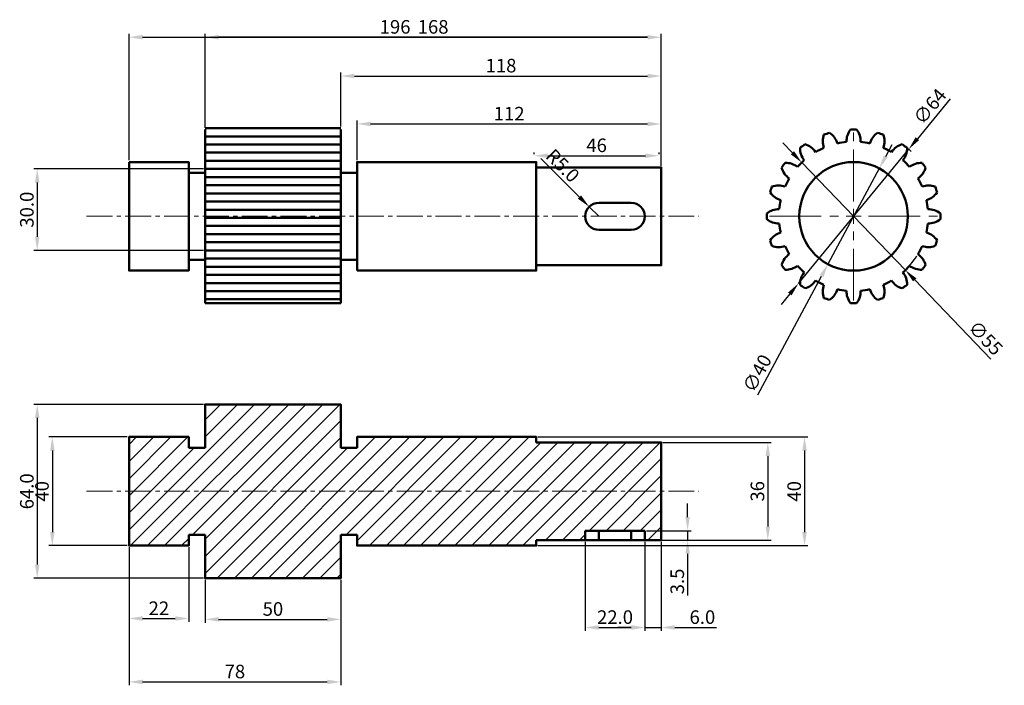
# Model space of a CAD drawing. Units: millimetres. Extents: x 2854 to 3217, y 1568 to 1813.
import ezdxf

# ---------------------------------------------------------------- set-up
doc = ezdxf.new("R2010")
doc.units = ezdxf.units.MM
doc.linetypes.add('CENTER2', pattern=[28.575, 19.05, -3.175, 3.175, -3.175])
for name, color, linetype, lineweight in [('M-CNTR', 1, 'CENTER2', 18), ('M-DIMS', 2, 'Continuous', 25), ('M-HATC', 8, 'Continuous', 18), ('M-OUTL', 7, 'Continuous', 50)]:
    doc.layers.add(name, color=color, linetype=linetype, lineweight=lineweight)
doc.styles.get("Standard").update_dxf_attribs({"font": 'arial.ttf'})
doc.dimstyles.new('ISO-25', dxfattribs={"dimtxt": 5, "dimasz": 5, "dimexe": 1.25, "dimexo": 0.625, "dimtad": 1, "dimdsep": 46, "dimtxsty": 'Standard', "dimcen": 2.5, "dimclrd": 3, "dimadec": 0, "dimazin": 0, "dimtfac": 1, "dimtmove": 0, "dimatfit": 3, "dimfxl": 1, "dimarcsym": 0})

# ---------------------------------------------------------------- blocks, each defined once
blk = doc.blocks.new('*D1')
at = {"layer": 'Defpoints', "color": 0, "transparency": 16777216}
for p in [(3090.59, 1806.21), (2894.59, 1760.27), (3090.59, 1758.27)]:
    blk.add_point(p, dxfattribs=at)
at = {"layer": 'M-DIMS', "color": 0, "lineweight": -2, "transparency": 16777216}
for p, q in [((2894.59, 1760.89), (2894.59, 1807.46)), ((2899.59, 1806.21), (3085.59, 1806.21)), ((3090.59, 1758.89), (3090.59, 1807.46))]:
    blk.add_line(p, q, dxfattribs=at)
at = {"layer": 'M-DIMS', "color": 0, "transparency": 16777216}
for points in [[(2899.59, 1807.05), (2899.59, 1805.38), (2894.59, 1806.21)], [(3085.59, 1807.05), (3085.59, 1805.38), (3090.59, 1806.21)]]:
    blk.add_solid(points, dxfattribs=at)
at = {"layer": 'M-DIMS', "color": 0, "transparency": 16777216, "insert": (2992.59, 1809.39), "char_height": 5, "attachment_point": 5}
blk.add_mtext('196', dxfattribs=at)
blk = doc.blocks.new('*D2')
at = {"layer": 'Defpoints', "color": 0, "transparency": 16777216}
for p in [(2922.59, 1806.21), (2922.59, 1772.27), (3090.59, 1758.27)]:
    blk.add_point(p, dxfattribs=at)
at = {"layer": 'M-DIMS', "color": 0, "lineweight": -2, "transparency": 16777216}
for p, q in [((2922.59, 1772.89), (2922.59, 1807.46)), ((3085.59, 1806.21), (2927.59, 1806.21)), ((3090.59, 1758.89), (3090.59, 1807.46))]:
    blk.add_line(p, q, dxfattribs=at)
at = {"layer": 'M-DIMS', "color": 0, "transparency": 16777216}
for points in [[(2927.59, 1807.05), (2927.59, 1805.38), (2922.59, 1806.21)], [(3085.59, 1807.05), (3085.59, 1805.38), (3090.59, 1806.21)]]:
    blk.add_solid(points, dxfattribs=at)
at = {"layer": 'M-DIMS', "color": 0, "transparency": 16777216, "insert": (3006.59, 1809.39), "char_height": 5, "attachment_point": 5}
blk.add_mtext('168', dxfattribs=at)
blk = doc.blocks.new('*D3')
at = {"layer": 'Defpoints', "color": 0, "transparency": 16777216}
for p in [(3090.59, 1791.93), (2972.59, 1772.72), (3090.59, 1772.72)]:
    blk.add_point(p, dxfattribs=at)
at = {"layer": 'M-DIMS', "color": 0, "lineweight": -2, "transparency": 16777216}
for p, q in [((2972.59, 1773.34), (2972.59, 1793.18)), ((2977.59, 1791.93), (3085.59, 1791.93)), ((3090.59, 1773.34), (3090.59, 1793.18))]:
    blk.add_line(p, q, dxfattribs=at)
at = {"layer": 'M-DIMS', "color": 0, "transparency": 16777216}
for points in [[(2977.59, 1792.77), (2977.59, 1791.1), (2972.59, 1791.93)], [(3085.59, 1792.77), (3085.59, 1791.1), (3090.59, 1791.93)]]:
    blk.add_solid(points, dxfattribs=at)
at = {"layer": 'M-DIMS', "color": 0, "transparency": 16777216, "insert": (3031.59, 1795.11), "char_height": 5, "attachment_point": 5}
blk.add_mtext('118', dxfattribs=at)
blk = doc.blocks.new('*D4')
at = {"layer": 'Defpoints', "color": 0, "transparency": 16777216}
for p in [(3090.59, 1774.28), (2978.59, 1760.27), (3090.59, 1760.27)]:
    blk.add_point(p, dxfattribs=at)
at = {"layer": 'M-DIMS', "color": 0, "lineweight": -2, "transparency": 16777216}
for p, q in [((2978.59, 1760.89), (2978.59, 1775.53)), ((2983.59, 1774.28), (3085.59, 1774.28)), ((3090.59, 1760.89), (3090.59, 1775.53))]:
    blk.add_line(p, q, dxfattribs=at)
at = {"layer": 'M-DIMS', "color": 0, "transparency": 16777216}
for points in [[(2983.59, 1775.12), (2983.59, 1773.45), (2978.59, 1774.28)], [(3085.59, 1775.12), (3085.59, 1773.45), (3090.59, 1774.28)]]:
    blk.add_solid(points, dxfattribs=at)
at = {"layer": 'M-DIMS', "color": 0, "transparency": 16777216, "insert": (3034.59, 1777.42), "char_height": 5, "attachment_point": 5}
blk.add_mtext('112', dxfattribs=at)
blk = doc.blocks.new('*D5')
at = {"layer": 'Defpoints', "color": 0, "transparency": 16777216}
for p in [(3043.81, 1762.58), (3089.81, 1762.58), (3089.81, 1762.58)]:
    blk.add_point(p, dxfattribs=at)
at = {"layer": 'M-DIMS', "color": 0, "lineweight": -2, "transparency": 16777216}
for p, q in [((3043.81, 1763.21), (3043.81, 1763.83)), ((3048.81, 1762.58), (3084.81, 1762.58)), ((3089.81, 1763.21), (3089.81, 1763.83))]:
    blk.add_line(p, q, dxfattribs=at)
at = {"layer": 'M-DIMS', "color": 0, "transparency": 16777216}
for points in [[(3048.81, 1763.42), (3048.81, 1761.75), (3043.81, 1762.58)], [(3084.81, 1763.42), (3084.81, 1761.75), (3089.81, 1762.58)]]:
    blk.add_solid(points, dxfattribs=at)
at = {"layer": 'M-DIMS', "color": 0, "transparency": 16777216, "insert": (3066.81, 1765.76), "char_height": 5, "attachment_point": 5}
blk.add_mtext('46', dxfattribs=at)
blk = doc.blocks.new('*D6')
at = {"layer": 'Defpoints', "color": 0, "transparency": 16777216}
for p in [(3181.76, 1765), (3141.14, 1715.54)]:
    blk.add_point(p, dxfattribs=at)
at = {"layer": 'M-DIMS', "color": 0, "lineweight": -2, "transparency": 16777216}
for p, q in [((3197, 1783.55), (3184.93, 1768.86)), ((3141.14, 1715.54), (3181.76, 1765)), ((3137.96, 1711.68), (3134.79, 1707.81))]:
    blk.add_line(p, q, dxfattribs=at)
blk.add_arc((3161.45, 1740.27), 32, 48.3615, 50.9227, dxfattribs=at)
at = {"layer": 'M-DIMS', "color": 0, "transparency": 16777216}
for points in [[(3184.29, 1769.39), (3185.58, 1768.33), (3181.76, 1765)], [(3137.32, 1712.21), (3138.61, 1711.15), (3141.14, 1715.54)]]:
    blk.add_solid(points, dxfattribs=at)
at = {"layer": 'M-DIMS', "color": 0, "transparency": 16777216, "insert": (3190.05, 1780.31), "char_height": 5, "attachment_point": 5, "rotation": 50.5996}
blk.add_mtext('∅64', dxfattribs=at)
blk = doc.blocks.new('*U7')
at = {"layer": 'M-CNTR', "color": 0, "transparency": 16777216}
for p, q in [((0, 5.5), (0, 31)), ((-31, 0), (-5.5, 0)), ((5.5, 0), (31, 0)), ((0, -31), (0, -5.5))]:
    blk.add_line(p, q, dxfattribs=at)
at = {"layer": 'M-CNTR', "color": 0, "linetype": 'Continuous', "transparency": 16777216}
for p, q in [((-2.75, 0), (2.75, 0)), ((0, -2.75), (0, 2.75))]:
    blk.add_line(p, q, dxfattribs=at)
blk = doc.blocks.new('*U8')
at = {"layer": 'M-CNTR', "color": 0, "transparency": 16777216}
for p, q in [((0, 5.5), (0, 31)), ((-31, 0), (-5.5, 0)), ((5.5, 0), (31, 0)), ((0, -31), (0, -5.5))]:
    blk.add_line(p, q, dxfattribs=at)
at = {"layer": 'M-CNTR', "color": 0, "linetype": 'Continuous', "transparency": 16777216}
for p, q in [((-2.75, 0), (2.75, 0)), ((0, -2.75), (0, 2.75))]:
    blk.add_line(p, q, dxfattribs=at)
blk = doc.blocks.new('*D9')
at = {"layer": 'Defpoints', "color": 0, "transparency": 16777216}
for p in [(3170.9, 1757.89), (3151.99, 1722.65)]:
    blk.add_point(p, dxfattribs=at)
at = {"layer": 'M-DIMS', "color": 0, "lineweight": -2, "transparency": 16777216}
for p, q in [((3173.27, 1762.3), (3175.63, 1766.71)), ((3170.9, 1757.89), (3151.99, 1722.65)), ((3126.17, 1674.51), (3149.63, 1718.24))]:
    blk.add_line(p, q, dxfattribs=at)
at = {"layer": 'M-DIMS', "color": 0, "transparency": 16777216}
for points in [[(3172.53, 1762.69), (3174, 1761.91), (3170.9, 1757.89)], [(3148.9, 1718.63), (3150.36, 1717.85), (3151.99, 1722.65)]]:
    blk.add_solid(points, dxfattribs=at)
at = {"layer": 'M-DIMS', "color": 0, "transparency": 16777216, "insert": (3126.52, 1682.17), "char_height": 5, "attachment_point": 5, "rotation": 61.7895}
blk.add_mtext('∅40', dxfattribs=at)
blk = doc.blocks.new('*D10')
at = {"layer": 'Defpoints', "color": 0, "transparency": 16777216}
for p in [(3142.37, 1760.08), (3180.52, 1720.46)]:
    blk.add_point(p, dxfattribs=at)
at = {"layer": 'M-DIMS', "color": 0, "lineweight": -2, "transparency": 16777216}
for p, q in [((3138.91, 1763.68), (3135.44, 1767.28)), ((3142.37, 1760.08), (3180.52, 1720.46)), ((3212.03, 1687.73), (3183.99, 1716.86))]:
    blk.add_line(p, q, dxfattribs=at)
blk.add_arc((3161.45, 1740.27), 27.5, 311.31, 328.1325, dxfattribs=at)
at = {"layer": 'M-DIMS', "color": 0, "transparency": 16777216}
for points in [[(3139.51, 1764.26), (3138.31, 1763.1), (3142.37, 1760.08)], [(3184.59, 1717.44), (3183.39, 1716.28), (3180.52, 1720.46)]]:
    blk.add_solid(points, dxfattribs=at)
at = {"layer": 'M-DIMS', "color": 0, "transparency": 16777216, "insert": (3209.61, 1695.03), "char_height": 5, "attachment_point": 5, "rotation": 313.9144}
blk.add_mtext('∅55', dxfattribs=at)
blk = doc.blocks.new('*D11')
at = {"layer": 'Defpoints', "color": 0, "transparency": 16777216}
for p in [(2894.59, 1659.01), (2866.36, 1619.01), (2894.59, 1619.01)]:
    blk.add_point(p, dxfattribs=at)
at = {"layer": 'M-DIMS', "color": 0, "lineweight": -2, "transparency": 16777216}
for p, q in [((2893.97, 1659.01), (2865.11, 1659.01)), ((2866.36, 1654.01), (2866.36, 1624.01)), ((2893.97, 1619.01), (2865.11, 1619.01))]:
    blk.add_line(p, q, dxfattribs=at)
at = {"layer": 'M-DIMS', "color": 0, "transparency": 16777216}
for points in [[(2865.52, 1654.01), (2867.19, 1654.01), (2866.36, 1659.01)], [(2865.52, 1624.01), (2867.19, 1624.01), (2866.36, 1619.01)]]:
    blk.add_solid(points, dxfattribs=at)
at = {"layer": 'M-DIMS', "color": 0, "transparency": 16777216, "insert": (2863.18, 1639.01), "char_height": 5, "attachment_point": 5, "rotation": 90}
blk.add_mtext('40', dxfattribs=at)
blk = doc.blocks.new('*D12')
at = {"layer": 'Defpoints', "color": 0, "transparency": 16777216}
for p in [(2894.59, 1619.01), (2916.59, 1619.01), (2916.59, 1592.18)]:
    blk.add_point(p, dxfattribs=at)
at = {"layer": 'M-DIMS', "color": 0, "lineweight": -2, "transparency": 16777216}
for p, q in [((2894.59, 1618.39), (2894.59, 1590.93)), ((2916.59, 1618.39), (2916.59, 1590.93)), ((2899.59, 1592.18), (2911.59, 1592.18))]:
    blk.add_line(p, q, dxfattribs=at)
at = {"layer": 'M-DIMS', "color": 0, "transparency": 16777216}
for points in [[(2899.59, 1593.01), (2899.59, 1591.34), (2894.59, 1592.18)], [(2911.59, 1593.01), (2911.59, 1591.34), (2916.59, 1592.18)]]:
    blk.add_solid(points, dxfattribs=at)
at = {"layer": 'M-DIMS', "color": 0, "transparency": 16777216, "insert": (2905.59, 1595.31), "char_height": 5, "attachment_point": 5}
blk.add_mtext('22', dxfattribs=at)
blk = doc.blocks.new('*D13')
at = {"layer": 'Defpoints', "color": 0, "transparency": 16777216}
for p in [(2922.59, 1607.01), (2972.59, 1607.01), (2972.59, 1591.86)]:
    blk.add_point(p, dxfattribs=at)
at = {"layer": 'M-DIMS', "color": 0, "lineweight": -2, "transparency": 16777216}
for p, q in [((2922.59, 1606.39), (2922.59, 1590.61)), ((2972.59, 1606.39), (2972.59, 1590.61)), ((2927.59, 1591.86), (2967.59, 1591.86))]:
    blk.add_line(p, q, dxfattribs=at)
at = {"layer": 'M-DIMS', "color": 0, "transparency": 16777216}
for points in [[(2927.59, 1592.69), (2927.59, 1591.03), (2922.59, 1591.86)], [(2967.59, 1592.69), (2967.59, 1591.03), (2972.59, 1591.86)]]:
    blk.add_solid(points, dxfattribs=at)
at = {"layer": 'M-DIMS', "color": 0, "transparency": 16777216, "insert": (2947.59, 1595.04), "char_height": 5, "attachment_point": 5}
blk.add_mtext('50', dxfattribs=at)
blk = doc.blocks.new('*D14')
at = {"layer": 'Defpoints', "color": 0, "transparency": 16777216}
for p in [(2894.59, 1597.47), (2972.59, 1597.47), (2972.59, 1568.83)]:
    blk.add_point(p, dxfattribs=at)
at = {"layer": 'M-DIMS', "color": 0, "lineweight": -2, "transparency": 16777216}
for p, q in [((2894.59, 1596.85), (2894.59, 1567.58)), ((2972.59, 1596.85), (2972.59, 1567.58)), ((2899.59, 1568.83), (2967.59, 1568.83))]:
    blk.add_line(p, q, dxfattribs=at)
at = {"layer": 'M-DIMS', "color": 0, "transparency": 16777216}
for points in [[(2899.59, 1569.66), (2899.59, 1567.99), (2894.59, 1568.83)], [(2967.59, 1569.66), (2967.59, 1567.99), (2972.59, 1568.83)]]:
    blk.add_solid(points, dxfattribs=at)
at = {"layer": 'M-DIMS', "color": 0, "transparency": 16777216, "insert": (2933.59, 1572.01), "char_height": 5, "attachment_point": 5}
blk.add_mtext('78', dxfattribs=at)
blk = doc.blocks.new('*D15')
at = {"layer": 'Defpoints', "color": 0, "transparency": 16777216}
for p in [(3090.59, 1657.01), (3090.59, 1621.01), (3129.86, 1621.01)]:
    blk.add_point(p, dxfattribs=at)
at = {"layer": 'M-DIMS', "color": 0, "lineweight": -2, "transparency": 16777216}
for p, q in [((3091.22, 1657.01), (3131.11, 1657.01)), ((3129.86, 1652.01), (3129.86, 1626.01)), ((3091.22, 1621.01), (3131.11, 1621.01))]:
    blk.add_line(p, q, dxfattribs=at)
at = {"layer": 'M-DIMS', "color": 0, "transparency": 16777216}
for points in [[(3129.02, 1652.01), (3130.69, 1652.01), (3129.86, 1657.01)], [(3129.02, 1626.01), (3130.69, 1626.01), (3129.86, 1621.01)]]:
    blk.add_solid(points, dxfattribs=at)
at = {"layer": 'M-DIMS', "color": 0, "transparency": 16777216, "insert": (3126.68, 1639.01), "char_height": 5, "attachment_point": 5, "rotation": 90}
blk.add_mtext('36', dxfattribs=at)
blk = doc.blocks.new('*D16')
at = {"layer": 'Defpoints', "color": 0, "transparency": 16777216}
for p in [(3044.59, 1659.01), (3044.59, 1619.01), (3143.4, 1619.01)]:
    blk.add_point(p, dxfattribs=at)
at = {"layer": 'M-DIMS', "color": 0, "lineweight": -2, "transparency": 16777216}
for p, q in [((3045.22, 1659.01), (3144.65, 1659.01)), ((3143.4, 1654.01), (3143.4, 1624.01)), ((3045.22, 1619.01), (3144.65, 1619.01))]:
    blk.add_line(p, q, dxfattribs=at)
at = {"layer": 'M-DIMS', "color": 0, "transparency": 16777216}
for points in [[(3142.56, 1654.01), (3144.23, 1654.01), (3143.4, 1659.01)], [(3142.56, 1624.01), (3144.23, 1624.01), (3143.4, 1619.01)]]:
    blk.add_solid(points, dxfattribs=at)
at = {"layer": 'M-DIMS', "color": 0, "transparency": 16777216, "insert": (3140.22, 1639.01), "char_height": 5, "attachment_point": 5, "rotation": 90}
blk.add_mtext('40', dxfattribs=at)
blk = doc.blocks.new('*D17')
at = {"layer": 'Defpoints', "color": 0, "transparency": 16777216}
for p in [(3084.59, 1624.51), (3084.59, 1621.01), (3100.33, 1621.01)]:
    blk.add_point(p, dxfattribs=at)
at = {"layer": 'M-DIMS', "color": 0, "lineweight": -2, "transparency": 16777216}
for p, q in [((3100.33, 1629.51), (3100.33, 1634.51)), ((3085.22, 1624.51), (3101.58, 1624.51)), ((3085.22, 1621.01), (3101.58, 1621.01)), ((3100.33, 1624.51), (3100.33, 1621.01)), ((3100.33, 1616.01), (3100.33, 1600.62))]:
    blk.add_line(p, q, dxfattribs=at)
at = {"layer": 'M-DIMS', "color": 0, "transparency": 16777216}
for points in [[(3099.49, 1629.51), (3101.16, 1629.51), (3100.33, 1624.51)], [(3099.49, 1616.01), (3101.16, 1616.01), (3100.33, 1621.01)]]:
    blk.add_solid(points, dxfattribs=at)
at = {"layer": 'M-DIMS', "color": 0, "transparency": 16777216, "insert": (3097.15, 1605.82), "char_height": 5, "attachment_point": 5, "rotation": 90}
blk.add_mtext('3.5', dxfattribs=at)
blk = doc.blocks.new('*D18')
at = {"layer": 'Defpoints', "color": 0, "transparency": 16777216}
for p in [(3062.59, 1621.01), (3084.59, 1621.01), (3084.59, 1588.86)]:
    blk.add_point(p, dxfattribs=at)
at = {"layer": 'M-DIMS', "color": 0, "lineweight": -2, "transparency": 16777216}
for p, q in [((3062.59, 1620.39), (3062.59, 1587.61)), ((3084.59, 1620.39), (3084.59, 1587.61))]:
    blk.add_line(p, q, dxfattribs=at)
at = {"layer": 'M-DIMS', "color": 3, "lineweight": -2, "transparency": 16777216}
blk.add_line((3067.59, 1588.86), (3079.59, 1588.86), dxfattribs=at)
at = {"layer": 'M-DIMS', "color": 3, "transparency": 16777216}
for points in [[(3067.59, 1589.7), (3067.59, 1588.03), (3062.59, 1588.86)], [(3079.59, 1589.7), (3079.59, 1588.03), (3084.59, 1588.86)]]:
    blk.add_solid(points, dxfattribs=at)
at = {"layer": 'M-DIMS', "color": 0, "transparency": 16777216, "insert": (3073.59, 1592.04), "char_height": 5, "attachment_point": 5}
blk.add_mtext('22.0', dxfattribs=at)
blk = doc.blocks.new('*D19')
at = {"layer": 'Defpoints', "color": 0, "transparency": 16777216}
for p in [(3084.59, 1621.01), (3090.59, 1621.01), (3090.59, 1588.86)]:
    blk.add_point(p, dxfattribs=at)
at = {"layer": 'M-DIMS', "color": 0, "lineweight": -2, "transparency": 16777216}
for p, q in [((3084.59, 1620.39), (3084.59, 1587.61)), ((3090.59, 1620.39), (3090.59, 1587.61))]:
    blk.add_line(p, q, dxfattribs=at)
at = {"layer": 'M-DIMS', "color": 3, "lineweight": -2, "transparency": 16777216}
for p, q in [((3079.59, 1588.86), (3074.59, 1588.86)), ((3084.59, 1588.86), (3090.59, 1588.86)), ((3095.59, 1588.86), (3110.96, 1588.86))]:
    blk.add_line(p, q, dxfattribs=at)
at = {"layer": 'M-DIMS', "color": 3, "transparency": 16777216}
for points in [[(3079.59, 1589.7), (3079.59, 1588.03), (3084.59, 1588.86)], [(3095.59, 1589.7), (3095.59, 1588.03), (3090.59, 1588.86)]]:
    blk.add_solid(points, dxfattribs=at)
at = {"layer": 'M-DIMS', "color": 0, "transparency": 16777216, "insert": (3105.77, 1592.04), "char_height": 5, "attachment_point": 5}
blk.add_mtext('6.0', dxfattribs=at)
blk = doc.blocks.new('*D20')
at = {"layer": 'Defpoints', "color": 0, "transparency": 16777216}
for p in [(2922.59, 1757.72), (2860.79, 1727.72), (2922.59, 1727.72)]:
    blk.add_point(p, dxfattribs=at)
at = {"layer": 'M-DIMS', "color": 0, "lineweight": -2, "transparency": 16777216}
for p, q in [((2921.97, 1757.72), (2859.54, 1757.72)), ((2921.97, 1727.72), (2859.54, 1727.72))]:
    blk.add_line(p, q, dxfattribs=at)
at = {"layer": 'M-DIMS', "color": 3, "lineweight": -2, "transparency": 16777216}
blk.add_line((2860.79, 1752.72), (2860.79, 1732.72), dxfattribs=at)
at = {"layer": 'M-DIMS', "color": 3, "transparency": 16777216}
for points in [[(2859.95, 1752.72), (2861.62, 1752.72), (2860.79, 1757.72)], [(2859.95, 1732.72), (2861.62, 1732.72), (2860.79, 1727.72)]]:
    blk.add_solid(points, dxfattribs=at)
at = {"layer": 'M-DIMS', "color": 0, "transparency": 16777216, "insert": (2857.61, 1742.72), "char_height": 5, "attachment_point": 5, "rotation": 90}
blk.add_mtext('30.0', dxfattribs=at)
blk = doc.blocks.new('*D21')
at = {"layer": 'Defpoints', "color": 0, "transparency": 16777216}
for p in [(2922.59, 1671.01), (2860.79, 1607.01), (2922.59, 1607.01)]:
    blk.add_point(p, dxfattribs=at)
at = {"layer": 'M-DIMS', "color": 0, "lineweight": -2, "transparency": 16777216}
for p, q in [((2921.97, 1671.01), (2859.54, 1671.01)), ((2921.97, 1607.01), (2859.54, 1607.01))]:
    blk.add_line(p, q, dxfattribs=at)
at = {"layer": 'M-DIMS', "color": 3, "lineweight": -2, "transparency": 16777216}
blk.add_line((2860.79, 1666.01), (2860.79, 1612.01), dxfattribs=at)
at = {"layer": 'M-DIMS', "color": 3, "transparency": 16777216}
for points in [[(2859.95, 1666.01), (2861.62, 1666.01), (2860.79, 1671.01)], [(2859.95, 1612.01), (2861.62, 1612.01), (2860.79, 1607.01)]]:
    blk.add_solid(points, dxfattribs=at)
at = {"layer": 'M-DIMS', "color": 0, "transparency": 16777216, "insert": (2857.61, 1639.01), "char_height": 5, "attachment_point": 5, "rotation": 90}
blk.add_mtext('64.0', dxfattribs=at)
blk = doc.blocks.new('*D22')
at = {"layer": 'Defpoints', "color": 0, "transparency": 16777216}
for p in [(3064.06, 1743.8), (3067.59, 1740.27)]:
    blk.add_point(p, dxfattribs=at)
at = {"layer": 'M-DIMS', "color": 3, "lineweight": -2, "transparency": 16777216}
for p, q in [((3046.29, 1761.57), (3060.52, 1747.34)), ((3067.59, 1740.27), (3064.06, 1743.8))]:
    blk.add_line(p, q, dxfattribs=at)
at = {"layer": 'M-DIMS', "color": 3, "transparency": 16777216}
blk.add_solid([(3061.11, 1747.93), (3059.93, 1746.75), (3064.06, 1743.8)], dxfattribs=at)
at = {"layer": 'M-DIMS', "color": 0, "transparency": 16777216, "insert": (3053.89, 1758.47), "char_height": 5, "attachment_point": 5, "rotation": 315.0014}
blk.add_mtext('R5.0', dxfattribs=at)

msp = doc.modelspace()

# ---------------------------------------------------------------- hatches: boundary and pattern name
at = {"layer": 'M-HATC'}
h = msp.add_hatch(dxfattribs=at)
h.set_pattern_fill('ANSI31', color=256, scale=1.4)
h.paths.add_polyline_path([(3062.593, 1621.012), (3062.593, 1624.512), (3084.593, 1624.512), (3084.593, 1621.012), (3090.593, 1621.012), (3090.593, 1657.012), (3044.593, 1657.012), (3044.593, 1659.012), (2978.593, 1659.012), (2978.593, 1655.012), (2972.593, 1655.012), (2972.593, 1671.012), (2922.593, 1671.012), (2922.593, 1655.012), (2916.593, 1655.012), (2916.593, 1659.012), (2894.593, 1659.012), (2894.593, 1619.012), (2916.593, 1619.012), (2916.593, 1623.012), (2922.593, 1623.012), (2922.593, 1607.012), (2972.593, 1607.012), (2972.593, 1623.012), (2978.593, 1623.012), (2978.593, 1619.012), (3044.593, 1619.012), (3044.593, 1621.012)])

# ---------------------------------------------------------------- linework, layer by layer
at = {"layer": 'M-CNTR', "ltscale": 0.5}
for p, q in [((2878.937, 1740.269), (3104.398, 1740.269)), ((2878.937, 1639.012), (3104.398, 1639.012))]:
    msp.add_line(p, q, dxfattribs=at)
at = {"layer": 'M-OUTL'}
for p, q in [((2922.593, 1772.716), (2972.593, 1772.716)), ((2922.593, 1708.269), (2922.593, 1772.269)), ((2922.593, 1769.716), (2972.593, 1769.716)), ((2972.593, 1772.269), (2972.593, 1708.269)), ((2922.593, 1766.716), (2972.593, 1766.716)), ((2922.593, 1763.716), (2972.593, 1763.716)), ((2922.593, 1760.716), (2972.593, 1760.716)), ((2922.593, 1757.716), (2972.593, 1757.716)), ((2922.593, 1754.716), (2972.593, 1754.716)), ((2922.593, 1751.716), (2972.593, 1751.716)), ((2922.593, 1748.716), (2972.593, 1748.716)), ((2922.593, 1745.716), (2972.593, 1745.716)), ((3067.593, 1745.269), (3079.593, 1745.269)), ((2922.593, 1742.716), (2972.593, 1742.716)), ((2922.593, 1739.716), (2972.593, 1739.716)), ((2922.593, 1736.716), (2972.593, 1736.716)), ((2922.593, 1733.716), (2972.593, 1733.716)), ((3067.593, 1735.269), (3079.593, 1735.269)), ((2922.593, 1730.716), (2972.593, 1730.716)), ((2922.593, 1727.716), (2972.593, 1727.716)), ((2922.593, 1724.716), (2972.593, 1724.716)), ((2922.593, 1721.716), (2972.593, 1721.716)), ((2922.593, 1718.716), (2972.593, 1718.716)), ((2922.593, 1715.716), (2972.593, 1715.716)), ((2922.593, 1712.716), (2972.593, 1712.716)), ((2922.593, 1709.716), (2972.593, 1709.716)), ((2972.593, 1708.269), (2922.593, 1708.269)), ((3084.593, 1624.512), (3062.593, 1624.512)), ((3062.593, 1624.512), (3062.593, 1621.012)), ((3067.593, 1621.012), (3067.593, 1624.512)), ((3079.507, 1624.512), (3079.507, 1621.012)), ((3084.593, 1621.012), (3084.593, 1624.512))]:
    msp.add_line(p, q, dxfattribs=at)
for points in [[(2894.593, 1760.269), (2916.593, 1760.269), (2916.593, 1720.269), (2894.593, 1720.269)], [(2978.593, 1720.269), (3044.593, 1720.269), (3044.593, 1760.269), (2978.593, 1760.269)], [(2916.593, 1756.269), (2922.593, 1756.269), (2922.593, 1724.269), (2916.593, 1724.269)], [(2972.593, 1756.269), (2978.593, 1756.269), (2978.593, 1724.269), (2972.593, 1724.269)], [(3044.593, 1722.269), (3090.593, 1722.269), (3090.593, 1758.269), (3044.593, 1758.269)]]:
    msp.add_lwpolyline(points, close=True, dxfattribs=at)
for points in [[(2922.593, 1655.012), (2922.593, 1671.012), (2972.593, 1671.012), (2972.593, 1655.012)], [(2916.593, 1623.012), (2916.593, 1619.012), (2894.593, 1619.012), (2894.593, 1659.012), (2916.593, 1659.012), (2916.593, 1655.012)], [(3044.593, 1657.012), (3044.593, 1659.012), (2978.593, 1659.012), (2978.593, 1655.012)], [(2916.593, 1655.012), (2922.593, 1655.012)], [(2972.593, 1655.012), (2978.593, 1655.012)], [(3044.593, 1621.012), (3090.593, 1621.012), (3090.593, 1657.012), (3044.593, 1657.012)], [(2922.593, 1623.012), (2916.593, 1623.012)], [(2972.593, 1623.012), (2972.593, 1607.012), (2922.593, 1607.012), (2922.593, 1623.012)], [(2978.593, 1623.012), (2972.593, 1623.012)], [(2978.593, 1623.012), (2978.593, 1619.012), (3044.593, 1619.012), (3044.593, 1621.012)]]:
    msp.add_lwpolyline(points, dxfattribs=at)
msp.add_circle((3161.448, 1740.269), 20, dxfattribs=at)
for centre, radius, start, end in [((3157.116, 1767.905), 7.028, 159.6648, 200.00243), ((3161.448, 1740.269), 32, 106.04172, 109.95828), ((3148.71, 1765.174), 7.028, 15.99757, 56.3352), ((3165.868, 1767.891), 7.028, 141.6648, 182.00243), ((3161.448, 1740.269), 32, 88.04172, 91.95828), ((3157.029, 1767.891), 7.028, 357.99757, 38.3352), ((3174.187, 1765.174), 7.028, 123.6648, 164.00243), ((3161.448, 1740.269), 32, 70.04172, 73.95828), ((3165.781, 1767.905), 7.028, 339.99757, 20.3352), ((3161.448, 1740.269), 32, 124.04172, 127.95828), ((3141.637, 1760.018), 7.028, 33.99757, 74.3352), ((3161.448, 1740.269), 27.5, 95.43463, 102.56537), ((3161.448, 1740.269), 27.5, 77.43463, 84.56537), ((3181.26, 1760.018), 7.028, 105.6648, 146.00243), ((3161.448, 1740.269), 32, 52.04172, 55.95828), ((3148.788, 1765.214), 7.028, 177.6648, 218.00243), ((3161.448, 1740.269), 27.5, 113.43463, 120.56537), ((3161.448, 1740.269), 27.5, 59.43463, 66.56537), ((3174.109, 1765.214), 7.028, 321.99757, 2.3352), ((3161.448, 1740.269), 32, 142.04172, 145.95828), ((3136.504, 1752.93), 7.028, 51.99757, 92.3352), ((3161.448, 1740.269), 27.5, 131.43463, 138.56537), ((3161.448, 1740.269), 27.5, 41.43463, 48.56537), ((3186.393, 1752.93), 7.028, 87.6648, 128.00243), ((3161.448, 1740.269), 32, 34.04172, 37.95828), ((3141.699, 1760.081), 7.028, 195.6648, 236.00243), ((3181.197, 1760.081), 7.028, 303.99757, 344.3352), ((3133.813, 1744.602), 7.028, 69.99757, 110.3352), ((3161.448, 1740.269), 27.5, 149.43463, 156.56537), ((3161.448, 1740.269), 27.5, 23.43463, 30.56537), ((3189.084, 1744.602), 7.028, 69.6648, 110.00243), ((3161.448, 1740.269), 32, 160.04172, 163.95828), ((3136.544, 1753.008), 7.028, 213.6648, 254.00243), ((3186.353, 1753.008), 7.028, 285.99757, 326.3352), ((3161.448, 1740.269), 32, 16.04172, 19.95828), ((3067.593, 1740.269), 5, 90, 270), ((3079.593, 1740.269), 5, 270, 90), ((3161.448, 1740.269), 27.5, 167.43463, 174.56537), ((3161.448, 1740.269), 27.5, 5.43463, 12.56537), ((3161.448, 1740.269), 32, 178.04172, 181.95828), ((3133.826, 1735.85), 7.028, 87.99757, 128.3352), ((3189.07, 1735.85), 7.028, 51.6648, 92.00243), ((3161.448, 1740.269), 32, 358.04172, 1.95828), ((3133.826, 1744.689), 7.028, 231.6648, 272.00243), ((3161.448, 1740.269), 27.5, 185.43463, 192.56537), ((3161.448, 1740.269), 27.5, 347.43463, 354.56537), ((3189.07, 1744.689), 7.028, 267.99757, 308.3352), ((3136.544, 1727.531), 7.028, 105.99757, 146.3352), ((3186.353, 1727.531), 7.028, 33.6648, 74.00243), ((3161.448, 1740.269), 32, 196.04172, 199.95828), ((3161.448, 1740.269), 32, 340.04172, 343.95828), ((3133.813, 1735.937), 7.028, 249.6648, 290.00243), ((3141.699, 1720.458), 7.028, 123.99757, 164.3352), ((3161.448, 1740.269), 27.5, 203.43463, 210.56537), ((3161.448, 1740.269), 27.5, 329.43463, 336.56537), ((3181.197, 1720.458), 7.028, 15.6648, 56.00243), ((3189.084, 1735.937), 7.028, 249.99757, 290.3352), ((3161.448, 1740.269), 32, 214.04172, 217.95828), ((3136.504, 1727.609), 7.028, 267.6648, 308.00243), ((3161.448, 1740.269), 27.5, 221.43463, 228.56537), ((3148.788, 1715.325), 7.028, 141.99757, 182.3352), ((3161.448, 1740.269), 27.5, 311.43463, 318.56537), ((3174.109, 1715.325), 7.028, 357.6648, 38.00243), ((3186.393, 1727.609), 7.028, 231.99757, 272.3352), ((3161.448, 1740.269), 32, 322.04172, 325.95828), ((3141.637, 1720.521), 7.028, 285.6648, 326.00243), ((3161.448, 1740.269), 27.5, 239.43463, 246.56537), ((3161.448, 1740.269), 27.5, 293.43463, 300.56537), ((3181.26, 1720.521), 7.028, 213.99757, 254.3352), ((3161.448, 1740.269), 32, 232.04172, 235.95828), ((3157.116, 1712.634), 7.028, 159.99757, 200.3352), ((3148.71, 1715.365), 7.028, 303.6648, 344.00243), ((3161.448, 1740.269), 27.5, 257.43463, 264.56537), ((3165.868, 1712.648), 7.028, 177.99757, 218.3352), ((3157.029, 1712.648), 7.028, 321.6648, 2.00243), ((3161.448, 1740.269), 27.5, 275.43463, 282.56537), ((3174.187, 1715.365), 7.028, 195.99757, 236.3352), ((3165.781, 1712.634), 7.028, 339.6648, 20.00243), ((3161.448, 1740.269), 32, 304.04172, 307.95828), ((3161.448, 1740.269), 32, 250.04172, 253.95828), ((3161.448, 1740.269), 32, 268.04172, 271.95828), ((3161.448, 1740.269), 32, 286.04172, 289.95828)]:
    msp.add_arc(centre, radius, start, end, dxfattribs=at)

# ---------------------------------------------------------------- block references
at = {"layer": 'M-CNTR'}
for name in ['*U7', '*U8']:
    msp.add_blockref(name, (3161.448, 1740.269), dxfattribs=at)

# ---------------------------------------------------------------- dimensions: what is measured, and where the dimension line sits
at = {"layer": 'M-DIMS'}
for base, p1, p2, override, picture, middle in [((3090.593, 1806.213), (2894.593, 1760.269), (3090.593, 1758.269), {"dimclrd": 0, "dimclre": 0, "dimclrt": 0}, '*D1', (2992.593, 1809.391)), ((2922.593, 1806.213), (3090.593, 1758.269), (2922.593, 1772.269), {"dimclrd": 0, "dimclre": 0, "dimclrt": 0, "dimtmove": 1}, '*D2', (3006.593, 1809.391)), ((3090.593, 1791.935), (2972.593, 1772.716), (3090.593, 1772.716), {"dimclrd": 0, "dimclre": 0, "dimclrt": 0}, '*D3', (3031.593, 1795.113)), ((3090.593, 1774.283), (2978.593, 1760.269), (3090.593, 1760.269), {"dimclrd": 0, "dimclre": 0, "dimclrt": 0}, '*D4', (3034.593, 1777.419)), ((3089.808, 1762.584), (3043.808, 1762.584), (3089.808, 1762.584), {"dimclrd": 0, "dimclre": 0, "dimclrt": 0}, '*D5', (3066.808, 1765.762)), ((3084.593, 1588.862), (3062.593, 1621.012), (3084.593, 1621.012), {"dimdec": 1, "dimlfac": 1, "dimrnd": 0, "dimzin": 0, "dimdsep": 46, "dimlunit": 2}, '*D18', (3073.593, 1592.04)), ((3090.593, 1588.862), (3084.593, 1621.012), (3090.593, 1621.012), {"dimdec": 1, "dimlfac": 1, "dimrnd": 0, "dimzin": 0, "dimdsep": 46, "dimlunit": 2}, '*D19', (3105.774, 1592.04)), ((2916.593, 1592.178), (2894.593, 1619.012), (2916.593, 1619.012), {"dimclrd": 0, "dimclre": 0, "dimclrt": 0}, '*D12', (2905.593, 1595.313)), ((2972.593, 1591.861), (2922.593, 1607.012), (2972.593, 1607.012), {"dimclrd": 0, "dimclre": 0, "dimclrt": 0}, '*D13', (2947.593, 1595.039)), ((2972.593, 1568.827), (2894.593, 1597.473), (2972.593, 1597.473), {"dimclrd": 0, "dimclre": 0, "dimclrt": 0}, '*D14', (2933.593, 1572.005))]:
    dim = msp.add_linear_dim(base=base, p1=p1, p2=p2, dimstyle='ISO-25', override=override, dxfattribs=at)
    dim.commit()
    dim.dimension.update_dxf_attribs({"geometry": picture, "text_midpoint": middle})
for p1, p2, picture, middle in [((3141.137, 1715.542), (3181.76, 1764.997), '*D6', (3192.61, 1778.206)), ((3170.903, 1757.894), (3151.994, 1722.645), '*D9', (3129.443, 1680.606)), ((3142.375, 1760.08), (3180.522, 1720.459), '*D10', (3207.217, 1692.732))]:
    dim = msp.add_diameter_dim_2p(p1=p1, p2=p2, dimstyle='ISO-25', override={"dimclrd": 0, "dimclre": 0, "dimclrt": 0}, dxfattribs=at)
    dim.commit()
    dim.dimension.update_dxf_attribs({"geometry": picture, "text_midpoint": middle, "dimtype": 163})
dim = msp.add_radius_dim(center=(3067.593, 1740.269), mpoint=(3064.057, 1743.805), dimstyle='ISO-25', override={"dimdec": 1, "dimlfac": 1, "dimrnd": 0, "dimzin": 0, "dimdsep": 46, "dimlunit": 2}, dxfattribs=at)
dim.commit()
dim.dimension.update_dxf_attribs({"geometry": '*D22', "text_midpoint": (3053.887, 1758.469)})
for base, p1, p2, override, picture, middle in [((2860.787, 1727.716), (2922.593, 1757.716), (2922.593, 1727.716), {"dimdec": 1, "dimlfac": 1, "dimrnd": 0, "dimzin": 0, "dimdsep": 46, "dimlunit": 2}, '*D20', (2857.608, 1742.716)), ((2860.787, 1607.012), (2922.593, 1671.012), (2922.593, 1607.012), {"dimdec": 1, "dimlfac": 1, "dimrnd": 0, "dimzin": 0, "dimdsep": 46, "dimlunit": 2}, '*D21', (2857.61, 1639.012)), ((2866.357, 1619.012), (2894.593, 1659.012), (2894.593, 1619.012), {"dimclrd": 0, "dimclre": 0, "dimclrt": 0}, '*D11', (2863.179, 1639.012)), ((3143.398, 1619.012), (3044.593, 1659.012), (3044.593, 1619.012), {"dimclrd": 0, "dimclre": 0, "dimclrt": 0}, '*D16', (3140.22, 1639.012)), ((3129.857, 1621.012), (3090.593, 1657.012), (3090.593, 1621.012), {"dimclrd": 0, "dimclre": 0, "dimclrt": 0}, '*D15', (3126.677, 1639.012)), ((3100.328, 1621.012), (3084.593, 1624.512), (3084.593, 1621.012), {"dimclrd": 0, "dimclre": 0, "dimclrt": 0}, '*D17', (3097.148, 1605.818))]:
    dim = msp.add_linear_dim(base=base, p1=p1, p2=p2, angle=90, dimstyle='ISO-25', override=override, dxfattribs=at)
    dim.commit()
    dim.dimension.update_dxf_attribs({"geometry": picture, "text_midpoint": middle})

doc.saveas('drawing.dxf')
